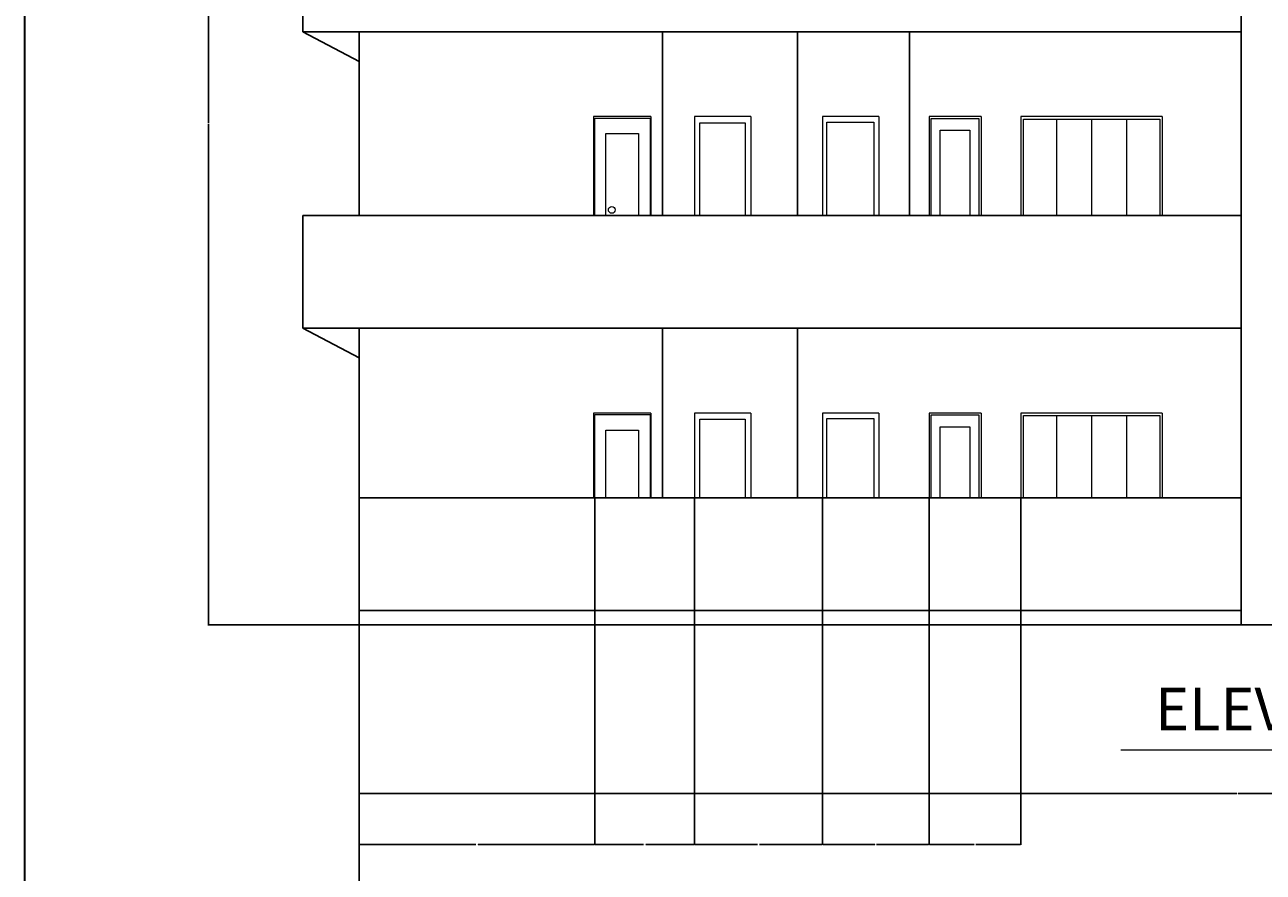
# Model space of a CAD drawing. Units: inches. Extents: x 2120 to 4013, y 1390 to 3019.
# Tile 47 of 59: x 2120 to 2647, y 2364 to 2724. Entities that reach past the tile are written whole.
import ezdxf

# ---------------------------------------------------------------- set-up
doc = ezdxf.new("R2010")
doc.units = ezdxf.units.IN
for name, color, linetype, lineweight in [('A-ANNO-DIMS', 2, 'Continuous', 18), ('A-ANNO-TEXT', 7, 'Continuous', 18), ('A-ANNO-TTLB', 7, 'Continuous', 35), ('A-DOOR', 3, 'Continuous', 18), ('A-ELEV', 7, 'Continuous', 25), ('A-GLAZ', 4, 'Continuous', 18), ('A-WALL-PATT', 252, 'Continuous', 13)]:
    doc.layers.add(name, color=color, linetype=linetype, lineweight=lineweight)
doc.styles.get("Standard").update_dxf_attribs({"font": 'arial.ttf'})
doc.dimstyles.get("Standard").update_dxf_attribs({"dimtxt": 0.18, "dimasz": 0.18, "dimexe": 0.18, "dimexo": 0.0625, "dimgap": 0.09, "dimtad": 0, "dimtih": 1, "dimtoh": 1, "dimdec": 4, "dimzin": 0, "dimdsep": 46, "dimtxsty": 'Standard', "dimcen": 0.09, "dimadec": 0, "dimazin": 0, "dimtfac": 1, "dimtdec": 4, "dimtofl": 0, "dimtmove": 0, "dimatfit": 3, "dimfxl": 1, "dimtolj": 1, "dimtzin": 0, "dimarcsym": 0})

# ---------------------------------------------------------------- blocks, each defined once
blk = doc.blocks.new('*D211')
at = {"layer": 'A-ANNO-DIMS', "color": 0, "lineweight": -2, "transparency": 16777216}
for p, q in [((2262.73, 2352.59), (2262.73, 2397.71)), ((2262.91, 2397.53), (2635.95, 2397.53)), ((3009.55, 2397.53), (2636.52, 2397.53)), ((3009.73, 2352.59), (3009.73, 2397.71))]:
    blk.add_line(p, q, dxfattribs=at)
at = {"layer": 'A-ANNO-DIMS', "color": 0, "transparency": 16777216}
for points in [[(2262.91, 2397.56), (2262.91, 2397.5), (2262.73, 2397.53)], [(3009.55, 2397.56), (3009.55, 2397.5), (3009.73, 2397.53)]]:
    blk.add_solid(points, dxfattribs=at)
at = {"layer": 'Defpoints', "color": 0, "transparency": 16777216}
for p in [(3009.73, 2397.53), (2262.73, 2352.53), (3009.73, 2352.53)]:
    blk.add_point(p, dxfattribs=at)
at = {"layer": 'A-ANNO-DIMS', "color": 0, "transparency": 16777216, "insert": (2636.23, 2397.53), "char_height": 0.18, "attachment_point": 5}
blk.add_mtext('\\A1;747', dxfattribs=at)
blk = doc.blocks.new('*D224')
at = {"layer": 'A-ANNO-DIMS', "color": 0, "lineweight": -2, "transparency": 16777216}
for p, q in [((2238.67, 2895.31), (2198.35, 2895.31)), ((2198.53, 2895.13), (2198.53, 2682.49)), ((2198.53, 2469.49), (2198.53, 2682.13)), ((2262.67, 2469.31), (2198.35, 2469.31))]:
    blk.add_line(p, q, dxfattribs=at)
at = {"layer": 'A-ANNO-DIMS', "color": 0, "transparency": 16777216}
for points in [[(2198.5, 2895.13), (2198.56, 2895.13), (2198.53, 2895.31)], [(2198.5, 2469.49), (2198.56, 2469.49), (2198.53, 2469.31)]]:
    blk.add_solid(points, dxfattribs=at)
at = {"layer": 'Defpoints', "color": 0, "transparency": 16777216}
for p in [(2198.53, 2895.31), (2238.73, 2895.31), (2262.73, 2469.31)]:
    blk.add_point(p, dxfattribs=at)
at = {"layer": 'A-ANNO-DIMS', "color": 0, "transparency": 16777216, "insert": (2198.53, 2682.31), "char_height": 0.18, "attachment_point": 5}
blk.add_mtext('\\A1;426', dxfattribs=at)
blk = doc.blocks.new('*D225')
at = {"layer": 'A-ANNO-DIMS', "color": 0, "lineweight": -2, "transparency": 16777216}
for p, q in [((2262.73, 2523.25), (2262.73, 2375.74)), ((2362.9, 2523.25), (2362.9, 2375.74)), ((2262.91, 2375.92), (2312.36, 2375.92)), ((2362.72, 2375.92), (2313.27, 2375.92))]:
    blk.add_line(p, q, dxfattribs=at)
at = {"layer": 'A-ANNO-DIMS', "color": 0, "transparency": 16777216}
for points in [[(2262.91, 2375.95), (2262.91, 2375.89), (2262.73, 2375.92)], [(2362.72, 2375.95), (2362.72, 2375.89), (2362.9, 2375.92)]]:
    blk.add_solid(points, dxfattribs=at)
at = {"layer": 'Defpoints', "color": 0, "transparency": 16777216}
for p in [(2262.73, 2523.31), (2362.9, 2523.31), (2362.9, 2375.92)]:
    blk.add_point(p, dxfattribs=at)
at = {"layer": 'A-ANNO-DIMS', "color": 0, "transparency": 16777216, "insert": (2312.82, 2375.92), "char_height": 0.18, "attachment_point": 5}
blk.add_mtext('\\A1;100.17', dxfattribs=at)
blk = doc.blocks.new('*D226')
at = {"layer": 'A-ANNO-DIMS', "color": 0, "lineweight": -2, "transparency": 16777216}
for p, q in [((2362.9, 2523.25), (2362.9, 2375.74)), ((2405.3, 2523.25), (2405.3, 2375.74)), ((2363.08, 2375.92), (2383.63, 2375.92)), ((2405.12, 2375.92), (2384.57, 2375.92))]:
    blk.add_line(p, q, dxfattribs=at)
at = {"layer": 'A-ANNO-DIMS', "color": 0, "transparency": 16777216}
for points in [[(2363.08, 2375.95), (2363.08, 2375.89), (2362.9, 2375.92)], [(2405.12, 2375.95), (2405.12, 2375.89), (2405.3, 2375.92)]]:
    blk.add_solid(points, dxfattribs=at)
at = {"layer": 'Defpoints', "color": 0, "transparency": 16777216}
for p in [(2362.9, 2523.31), (2405.3, 2523.31), (2405.3, 2375.92)]:
    blk.add_point(p, dxfattribs=at)
at = {"layer": 'A-ANNO-DIMS', "color": 0, "transparency": 16777216, "insert": (2384.1, 2375.92), "char_height": 0.18, "attachment_point": 5}
blk.add_mtext('\\A1;42.404', dxfattribs=at)
blk = doc.blocks.new('*D227')
at = {"layer": 'A-ANNO-DIMS', "color": 0, "lineweight": -2, "transparency": 16777216}
for p, q in [((2405.3, 2523.25), (2405.3, 2375.74)), ((2459.67, 2523.25), (2459.67, 2375.74)), ((2405.48, 2375.92), (2432.09, 2375.92)), ((2459.49, 2375.92), (2432.88, 2375.92))]:
    blk.add_line(p, q, dxfattribs=at)
at = {"layer": 'A-ANNO-DIMS', "color": 0, "transparency": 16777216}
for points in [[(2405.48, 2375.95), (2405.48, 2375.89), (2405.3, 2375.92)], [(2459.49, 2375.95), (2459.49, 2375.89), (2459.67, 2375.92)]]:
    blk.add_solid(points, dxfattribs=at)
at = {"layer": 'Defpoints', "color": 0, "transparency": 16777216}
for p in [(2405.3, 2523.31), (2459.67, 2523.31), (2459.67, 2375.92)]:
    blk.add_point(p, dxfattribs=at)
at = {"layer": 'A-ANNO-DIMS', "color": 0, "transparency": 16777216, "insert": (2432.49, 2375.92), "char_height": 0.18, "attachment_point": 5}
blk.add_mtext('\\A1;54.37', dxfattribs=at)
blk = doc.blocks.new('*D228')
at = {"layer": 'A-ANNO-DIMS', "color": 0, "lineweight": -2, "transparency": 16777216}
for p, q in [((2459.67, 2523.25), (2459.67, 2375.74)), ((2505.02, 2523.25), (2505.02, 2375.74)), ((2459.85, 2375.92), (2481.95, 2375.92)), ((2504.84, 2375.92), (2482.74, 2375.92))]:
    blk.add_line(p, q, dxfattribs=at)
at = {"layer": 'A-ANNO-DIMS', "color": 0, "transparency": 16777216}
for points in [[(2459.85, 2375.95), (2459.85, 2375.89), (2459.67, 2375.92)], [(2504.84, 2375.95), (2504.84, 2375.89), (2505.02, 2375.92)]]:
    blk.add_solid(points, dxfattribs=at)
at = {"layer": 'Defpoints', "color": 0, "transparency": 16777216}
for p in [(2459.67, 2523.31), (2505.02, 2523.31), (2505.02, 2375.92)]:
    blk.add_point(p, dxfattribs=at)
at = {"layer": 'A-ANNO-DIMS', "color": 0, "transparency": 16777216, "insert": (2482.34, 2375.92), "char_height": 0.18, "attachment_point": 5}
blk.add_mtext('\\A1;45.35', dxfattribs=at)
blk = doc.blocks.new('*D229')
at = {"layer": 'A-ANNO-DIMS', "color": 0, "lineweight": -2, "transparency": 16777216}
for p, q in [((2505.02, 2523.25), (2505.02, 2375.74)), ((2544.14, 2523.25), (2544.14, 2375.74)), ((2505.2, 2375.92), (2524.19, 2375.92)), ((2543.96, 2375.92), (2524.97, 2375.92))]:
    blk.add_line(p, q, dxfattribs=at)
at = {"layer": 'A-ANNO-DIMS', "color": 0, "transparency": 16777216}
for points in [[(2505.2, 2375.95), (2505.2, 2375.89), (2505.02, 2375.92)], [(2543.96, 2375.95), (2543.96, 2375.89), (2544.14, 2375.92)]]:
    blk.add_solid(points, dxfattribs=at)
at = {"layer": 'Defpoints', "color": 0, "transparency": 16777216}
for p in [(2505.02, 2523.31), (2544.14, 2523.31), (2544.14, 2375.92)]:
    blk.add_point(p, dxfattribs=at)
at = {"layer": 'A-ANNO-DIMS', "color": 0, "transparency": 16777216, "insert": (2524.58, 2375.92), "char_height": 0.18, "attachment_point": 5}
blk.add_mtext('\\A1;39.12', dxfattribs=at)

msp = doc.modelspace()

# ---------------------------------------------------------------- hatches: boundary and pattern name
at = {"layer": 'A-WALL-PATT'}
h = msp.add_hatch(dxfattribs=at)
h.set_pattern_fill('ANSI32', color=256)
h.paths.add_polyline_path([(2271.7331, 2343.531), (2283.3788, 2343.531), (2283.3788, 2348.031), (2283.3788, 2352.5306), (2262.7331, 2352.5306), (2262.7331, 2182.638), (2267.2331, 2182.638), (2271.7331, 2182.638), (2271.7331, 2219.031), (2391.7331, 2219.031), (2391.7331, 2214.189), (2393.9831, 2214.189), (2396.2331, 2214.189), (2396.2331, 2219.031), (2420.2331, 2219.031), (2420.2331, 2225.7535), (2417.2197, 2225.7535), (2415.7331, 2225.7535), (2415.7331, 2223.5306), (2271.7331, 2223.5306)])
h.paths.add_polyline_path([(2380.0942, 2352.5306), (2343.3788, 2352.5306), (2343.3788, 2343.531), (2363.2331, 2343.531), (2363.2331, 2288.8489), (2365.4831, 2288.8489), (2367.7331, 2288.8489), (2367.7331, 2343.531), (2380.0942, 2343.531)], flags=17)
h.paths.add_polyline_path([(2432.4339, 2352.5306), (2404.0943, 2352.5306), (2404.0943, 2343.531), (2415.7331, 2343.531), (2415.7331, 2264.0306), (2367.7331, 2264.0306), (2367.7331, 2266.4872), (2363.2331, 2266.4872), (2363.2331, 2259.531), (2367.7331, 2259.531), (2415.7331, 2259.531), (2415.7331, 2255.0658), (2420.2331, 2255.0658), (2420.2331, 2259.531), (2424.5717, 2259.531), (2424.5717, 2261.781), (2424.5717, 2264.0306), (2420.2331, 2264.0306), (2420.2331, 2343.531), (2432.4339, 2343.531)])
h.paths.add_polyline_path([(2508.9115, 2352.5306), (2456.4339, 2352.5306), (2456.4339, 2343.531), (2468.2331, 2343.531), (2468.2331, 2264.0306), (2448.0487, 2264.0306), (2448.0487, 2259.531), (2468.2331, 2259.531), (2468.2331, 2255.5496), (2472.7331, 2255.5496), (2472.7331, 2343.531), (2508.9115, 2343.531)])
h.paths.add_polyline_path([(2637.7331, 2352.5306), (2544.9116, 2352.5306), (2544.9116, 2343.531), (2589.7331, 2343.531), (2633.2331, 2343.531), (2637.7331, 2343.531)])
h.paths.add_polyline_path([(2594.2331, 2343.5306), (2589.7331, 2343.5306), (2589.7331, 2259.5306), (2589.7331, 2252.4915), (2591.9831, 2252.4915), (2594.2331, 2252.4915)])
h.paths.add_polyline_path([(2637.7331, 2223.5306), (2594.2331, 2223.5306), (2594.2331, 2230.1988), (2591.9831, 2230.1988), (2589.7331, 2230.1988), (2589.7331, 2223.5306), (2472.7331, 2223.5306), (2468.2331, 2223.5306), (2468.2331, 2219.031), (2628.7331, 2219.031), (2628.7331, 2138.031), (2637.7331, 2138.031)])
h.paths.add_polyline_path([(3822.6535, 2458.4402), (3874.9468, 2458.4402), (3874.9468, 2476.9866), (3822.6535, 2476.9866)], flags=9)
h.paths.add_polyline_path([(3834.6921, 2781.8174), (3935.9206, 2781.8174), (3935.9206, 2800.3638), (3834.6921, 2800.3638)], flags=9)
h.paths.add_polyline_path([(3832.2843, 2837.9683), (3884.5776, 2837.9683), (3884.5776, 2856.5146), (3832.2843, 2856.5146)], flags=9)
h.paths.add_polyline_path([(3830.9388, 2861.4782), (3956.8958, 2861.4782), (3956.8958, 2880.0245), (3830.9388, 2880.0245)], flags=9)
h.paths.add_polyline_path([(3870.6966, 2352.5752), (3887.9272, 2352.5752), (3887.9272, 2377.3037), (3870.6966, 2377.3037)], flags=9)
h.paths.add_polyline_path([(3289.2701, 2413.161), (3435.2223, 2413.161), (3435.2223, 2450.2538), (3289.2701, 2450.2538)], flags=9)
h.paths.add_polyline_path([(2487.6944, 2414.3601), (2637.8335, 2414.3601), (2637.8335, 2451.4528), (2487.6944, 2451.4528)], flags=9)
h.paths.add_polyline_path([(2567.3724, 1457.9199), (2815.296, 1457.9199), (2815.296, 1495.0127), (2567.3724, 1495.0127)], flags=9)
h.paths.add_polyline_path([(2655.3825, 2093.2363), (2685.9555, 2093.2363), (2685.9555, 2111.8937), (2655.3825, 2111.8937)], flags=9)
h.paths.add_polyline_path([(2543.9218, 1550.6671), (2587.8406, 1550.6671), (2587.8406, 1569.3244), (2543.9218, 1569.3244)], flags=9)
h.paths.add_polyline_path([(2905.1384, 1543.8113), (2949.0572, 1543.8113), (2949.0572, 1562.4686), (2905.1384, 1562.4686)], flags=9)
h.paths.add_polyline_path([(2736.4118, 1702.4736), (2784.2153, 1702.4736), (2784.2153, 1721.1309), (2736.4118, 1721.1309)], flags=9)
h.paths.add_polyline_path([(2912.8666, 1710.4168), (2951.707, 1710.4168), (2951.707, 1729.0741), (2912.8666, 1729.0741)], flags=9)
h.paths.add_polyline_path([(2923.5785, 1763.5038), (2959.7279, 1763.5038), (2959.7279, 1782.1611), (2923.5785, 1782.1611)], flags=9)
h.paths.add_polyline_path([(2925.2114, 1809.6137), (2967.1861, 1809.6137), (2967.1861, 1828.271), (2925.2114, 1828.271)], flags=9)
h.paths.add_polyline_path([(2996.2711, 1878.9003), (2996.2711, 1913.109), (2977.6138, 1913.109), (2977.6138, 1878.9003)], flags=9)
h.paths.add_polyline_path([(2883.0859, 1895.7192), (2927.1855, 1895.7192), (2927.1855, 1914.3766), (2883.0859, 1914.3766)], flags=9)
h.paths.add_polyline_path([(2787.3924, 1810.8013), (2841.0213, 1810.8013), (2841.0213, 1829.4587), (2787.3924, 1829.4587)], flags=9)
h.paths.add_polyline_path([(2775.6399, 2101.7395), (2829.2689, 2101.7395), (2829.2689, 2120.3968), (2775.6399, 2120.3968)], flags=9)
h.paths.add_polyline_path([(2913.0263, 2075.817), (2951.8667, 2075.817), (2951.8667, 2094.4744), (2913.0263, 2094.4744)], flags=9)
h.paths.add_polyline_path([(2929.966, 2133.3669), (2966.1154, 2133.3669), (2966.1154, 2152.0243), (2929.966, 2152.0243)], flags=9)
h.paths.add_polyline_path([(2932.7502, 2182.6088), (2968.8996, 2182.6088), (2968.8996, 2201.2662), (2932.7502, 2201.2662)], flags=9)
h.paths.add_polyline_path([(2996.0681, 2266.3173), (2996.0681, 2300.5261), (2977.4108, 2300.5261), (2977.4108, 2266.3173)], flags=9)
h.paths.add_polyline_path([(2885.1039, 2279.2186), (2929.2035, 2279.2186), (2929.2035, 2297.8759), (2885.1039, 2297.8759)], flags=9)
h.paths.add_polyline_path([(2735.7042, 2218.3197), (2783.5078, 2218.3197), (2783.5078, 2236.9771), (2735.7042, 2236.9771)], flags=9)
h.paths.add_polyline_path([(2635.6049, 2044.0085), (2648.9678, 2044.0085), (2648.9678, 2054.312), (2635.6049, 2054.312)], flags=9)
h.paths.add_polyline_path([(2714.0148, 1923.0473), (2727.3777, 1923.0473), (2727.3777, 1933.3508), (2714.0148, 1933.3508)], flags=9)
h.paths.add_polyline_path([(2709.0345, 1988.1628), (2722.3974, 1988.1628), (2722.3974, 1998.4663), (2709.0345, 1998.4663)], flags=9)
h.paths.add_polyline_path([(2592.8935, 1962.1763), (2606.2564, 1962.1763), (2606.2564, 1972.4799), (2592.8935, 1972.4799)], flags=9)
h.paths.add_polyline_path([(2618.3996, 1985.9724), (2644.1942, 1985.9724), (2644.1942, 1996.2759), (2618.3996, 1996.2759)], flags=9)
h.paths.add_polyline_path([(2601.279, 1920.5869), (2614.6419, 1920.5869), (2614.6419, 1930.8904), (2601.279, 1930.8904)], flags=9)
h.paths.add_polyline_path([(2692.3278, 1932.7645), (2704.5311, 1932.7645), (2704.5311, 1943.0681), (2692.3278, 1943.0681)], flags=9)
h.paths.add_polyline_path([(2311.122, 1672.7318), (2355.0408, 1672.7318), (2355.0408, 1691.3892), (2311.122, 1691.3892)], flags=9)
h.paths.add_polyline_path([(2456.2551, 1632.3198), (2492.4796, 1632.3198), (2492.4796, 1650.9772), (2456.2551, 1650.9772)], flags=9)
h.paths.add_polyline_path([(2401.0766, 1631.4793), (2437.301, 1631.4793), (2437.301, 1650.1367), (2401.0766, 1650.1367)], flags=9)
h.paths.add_polyline_path([(2546.7054, 1700.9235), (2594.509, 1700.9235), (2594.509, 1719.5809), (2546.7054, 1719.5809)], flags=9)
h.paths.add_polyline_path([(2445.4866, 1766.9937), (2497.5261, 1766.9937), (2497.5261, 1785.651), (2445.4866, 1785.651)], flags=9)
h.paths.add_polyline_path([(2287.9992, 1739.7675), (2326.8396, 1739.7675), (2326.8396, 1758.4248), (2287.9992, 1758.4248)], flags=9)
h.paths.add_polyline_path([(2458.5279, 1924.7607), (2510.5675, 1924.7607), (2510.5675, 1943.4181), (2458.5279, 1943.4181)], flags=9)
h.paths.add_polyline_path([(2309.2811, 1902.7642), (2345.4305, 1902.7642), (2345.4305, 1921.4215), (2309.2811, 1921.4215)], flags=9)
h.paths.add_polyline_path([(2490.7554, 2018.9392), (2530.7896, 2018.9392), (2530.7896, 2037.5965), (2490.7554, 2037.5965)], flags=9)
h.paths.add_polyline_path([(2402.143, 2024.7393), (2438.5414, 2024.7393), (2438.5414, 2043.3966), (2402.143, 2043.3966)], flags=9)
h.paths.add_polyline_path([(2287.856, 1931.7926), (2326.6964, 1931.7926), (2326.6964, 1950.4499), (2287.856, 1950.4499)], flags=9)
h.paths.add_polyline_path([(2281.7979, 2193.5771), (2320.6383, 2193.5771), (2320.6383, 2212.2344), (2281.7979, 2212.2344)], flags=25)
h.paths.add_polyline_path([(2484.0754, 2093.892), (2536.115, 2093.892), (2536.115, 2112.5494), (2484.0754, 2112.5494)], flags=9)
h.paths.add_polyline_path([(2624.7948, 2281.8639), (2624.7948, 2311.4137), (2606.1375, 2311.4137), (2606.1375, 2281.8639)], flags=9)
h.paths.add_polyline_path([(2507.5036, 2290.3639), (2541.934, 2290.3639), (2541.934, 2309.0212), (2507.5036, 2309.0212)], flags=9)
h.paths.add_polyline_path([(2423.1076, 2285.2202), (2459.332, 2285.2202), (2459.332, 2303.8776), (2423.1076, 2303.8776)], flags=9)
h.paths.add_polyline_path([(2374.5467, 2289.6272), (2410.7711, 2289.6272), (2410.7711, 2308.2846), (2374.5467, 2308.2846)], flags=25)
h.paths.add_polyline_path([(2277.4907, 2227.5651), (2316.3311, 2227.5651), (2316.3311, 2246.2224), (2277.4907, 2246.2224)], flags=25)
h.paths.add_polyline_path([(2655.3825, 2093.2367), (2685.9555, 2093.2367), (2685.9555, 2111.894), (2655.3825, 2111.894)], flags=9)
h.paths.add_polyline_path([(2543.9217, 1550.6674), (2587.8406, 1550.6674), (2587.8406, 1569.3247), (2543.9217, 1569.3247)], flags=9)
h.paths.add_polyline_path([(2905.1384, 1543.8116), (2949.0572, 1543.8116), (2949.0572, 1562.4689), (2905.1384, 1562.4689)], flags=9)
h.paths.add_polyline_path([(2736.4118, 1702.4739), (2784.2153, 1702.4739), (2784.2153, 1721.1312), (2736.4118, 1721.1312)], flags=9)
h.paths.add_polyline_path([(2912.8666, 1710.4171), (2951.707, 1710.4171), (2951.707, 1729.0744), (2912.8666, 1729.0744)], flags=9)
h.paths.add_polyline_path([(2923.5785, 1763.5041), (2959.7279, 1763.5041), (2959.7279, 1782.1614), (2923.5785, 1782.1614)], flags=9)
h.paths.add_polyline_path([(2925.2114, 1809.614), (2967.1861, 1809.614), (2967.1861, 1828.2713), (2925.2114, 1828.2713)], flags=9)
h.paths.add_polyline_path([(2996.2711, 1878.9006), (2996.2711, 1913.1094), (2977.6137, 1913.1094), (2977.6137, 1878.9006)], flags=9)
h.paths.add_polyline_path([(2883.0859, 1895.7195), (2927.1855, 1895.7195), (2927.1855, 1914.3769), (2883.0859, 1914.3769)], flags=9)
h.paths.add_polyline_path([(2787.3924, 1810.8016), (2841.0213, 1810.8016), (2841.0213, 1829.459), (2787.3924, 1829.459)], flags=9)
h.paths.add_polyline_path([(2775.6399, 2101.7398), (2829.2688, 2101.7398), (2829.2688, 2120.3971), (2775.6399, 2120.3971)], flags=9)
h.paths.add_polyline_path([(2913.0263, 2075.8173), (2951.8667, 2075.8173), (2951.8667, 2094.4747), (2913.0263, 2094.4747)], flags=9)
h.paths.add_polyline_path([(2929.966, 2133.3672), (2966.1154, 2133.3672), (2966.1154, 2152.0246), (2929.966, 2152.0246)], flags=9)
h.paths.add_polyline_path([(2932.7502, 2182.6091), (2968.8996, 2182.6091), (2968.8996, 2201.2665), (2932.7502, 2201.2665)], flags=9)
h.paths.add_polyline_path([(2996.0681, 2266.3176), (2996.0681, 2300.5264), (2977.4108, 2300.5264), (2977.4108, 2266.3176)], flags=9)
h.paths.add_polyline_path([(2885.1039, 2279.2189), (2929.2035, 2279.2189), (2929.2035, 2297.8762), (2885.1039, 2297.8762)], flags=9)
h.paths.add_polyline_path([(2735.7042, 2218.32), (2783.5078, 2218.32), (2783.5078, 2236.9774), (2735.7042, 2236.9774)], flags=9)
h.paths.add_polyline_path([(2635.6048, 2044.0088), (2648.9677, 2044.0088), (2648.9677, 2054.3123), (2635.6048, 2054.3123)], flags=9)
h.paths.add_polyline_path([(2714.0148, 1923.0476), (2727.3777, 1923.0476), (2727.3777, 1933.3511), (2714.0148, 1933.3511)], flags=9)
h.paths.add_polyline_path([(2709.0345, 1988.1631), (2722.3974, 1988.1631), (2722.3974, 1998.4666), (2709.0345, 1998.4666)], flags=9)
h.paths.add_polyline_path([(2592.8935, 1962.1766), (2606.2564, 1962.1766), (2606.2564, 1972.4802), (2592.8935, 1972.4802)], flags=9)
h.paths.add_polyline_path([(2618.3995, 1985.9727), (2644.1942, 1985.9727), (2644.1942, 1996.2762), (2618.3995, 1996.2762)], flags=9)
h.paths.add_polyline_path([(2601.279, 1920.5872), (2614.6419, 1920.5872), (2614.6419, 1930.8908), (2601.279, 1930.8908)], flags=9)
h.paths.add_polyline_path([(2692.3278, 1932.7648), (2704.5311, 1932.7648), (2704.5311, 1943.0684), (2692.3278, 1943.0684)], flags=9)
h.paths.add_polyline_path([(2311.122, 1672.7321), (2355.0408, 1672.7321), (2355.0408, 1691.3895), (2311.122, 1691.3895)], flags=9)
h.paths.add_polyline_path([(2456.2551, 1632.3201), (2492.4795, 1632.3201), (2492.4795, 1650.9775), (2456.2551, 1650.9775)], flags=9)
h.paths.add_polyline_path([(2401.0766, 1631.4796), (2437.301, 1631.4796), (2437.301, 1650.137), (2401.0766, 1650.137)], flags=9)
h.paths.add_polyline_path([(2546.7054, 1700.9238), (2594.509, 1700.9238), (2594.509, 1719.5812), (2546.7054, 1719.5812)], flags=9)
h.paths.add_polyline_path([(2445.4866, 1766.994), (2497.5261, 1766.994), (2497.5261, 1785.6513), (2445.4866, 1785.6513)], flags=9)
h.paths.add_polyline_path([(2287.9992, 1739.7678), (2326.8396, 1739.7678), (2326.8396, 1758.4251), (2287.9992, 1758.4251)], flags=9)
h.paths.add_polyline_path([(2458.5279, 1924.7611), (2510.5675, 1924.7611), (2510.5675, 1943.4184), (2458.5279, 1943.4184)], flags=9)
h.paths.add_polyline_path([(2309.2811, 1902.7645), (2345.4305, 1902.7645), (2345.4305, 1921.4218), (2309.2811, 1921.4218)], flags=9)
h.paths.add_polyline_path([(2490.7554, 2018.9395), (2530.7895, 2018.9395), (2530.7895, 2037.5968), (2490.7554, 2037.5968)], flags=9)
h.paths.add_polyline_path([(2402.143, 2024.7396), (2438.5413, 2024.7396), (2438.5413, 2043.3969), (2402.143, 2043.3969)], flags=9)
h.paths.add_polyline_path([(2287.856, 1931.7929), (2326.6964, 1931.7929), (2326.6964, 1950.4502), (2287.856, 1950.4502)], flags=9)
h.paths.add_polyline_path([(2281.7979, 2193.5774), (2320.6383, 2193.5774), (2320.6383, 2212.2347), (2281.7979, 2212.2347)], flags=25)
h.paths.add_polyline_path([(2484.0754, 2093.8924), (2536.115, 2093.8924), (2536.115, 2112.5497), (2484.0754, 2112.5497)], flags=9)
h.paths.add_polyline_path([(2624.7948, 2281.8642), (2624.7948, 2311.414), (2606.1374, 2311.414), (2606.1374, 2281.8642)], flags=9)
h.paths.add_polyline_path([(2507.5035, 2290.3642), (2541.934, 2290.3642), (2541.934, 2309.0215), (2507.5035, 2309.0215)], flags=9)
h.paths.add_polyline_path([(2423.1075, 2285.2205), (2459.332, 2285.2205), (2459.332, 2303.8779), (2423.1075, 2303.8779)], flags=9)
h.paths.add_polyline_path([(2374.5467, 2289.6275), (2410.7711, 2289.6275), (2410.7711, 2308.2849), (2374.5467, 2308.2849)], flags=25)
h.paths.add_polyline_path([(2277.4907, 2227.5654), (2316.3311, 2227.5654), (2316.3311, 2246.2227), (2277.4907, 2246.2227)], flags=25)
h = msp.add_hatch(dxfattribs=at)
h.set_pattern_fill('ANSI32', color=256)
h.paths.add_polyline_path([(2271.7331, 1980.389), (2262.7331, 1980.389), (2262.7331, 1912.8434), (2267.2331, 1912.8434), (2271.7331, 1912.8434), (2271.7331, 1922.531), (2351.2331, 1922.531), (2351.2331, 1901.4728), (2355.7331, 1901.4728), (2355.7331, 1922.531), (2357.9815, 1922.531), (2357.9815, 1926.5306), (2271.7331, 1926.5306)])
h.paths.add_polyline_path([(2589.2331, 1949.1622), (2584.7331, 1949.1622), (2580.2331, 1949.1622), (2580.2331, 1874.5306), (2355.7331, 1874.5306), (2355.7331, 1880.1922), (2351.2331, 1880.1922), (2351.2331, 1874.5306), (2271.7331, 1874.5306), (2271.7331, 1888.8431), (2262.7331, 1888.8431), (2262.7331, 1842.2909), (2267.2331, 1842.2909), (2271.7331, 1842.2909), (2271.7331, 1865.531), (2415.7331, 1865.531), (2415.7331, 1779.7286), (2420.2331, 1779.7286), (2420.2331, 1865.531), (2589.2331, 1865.531)])
h.paths.add_polyline_path([(2271.7331, 1782.2906), (2262.7331, 1782.2906), (2262.7331, 1711.4639), (2267.2331, 1711.4639), (2271.7331, 1711.4639), (2271.7331, 1738.031), (2420.2331, 1738.031), (2420.2331, 1742.531), (2420.2331, 1747.3376), (2417.9831, 1747.3376), (2415.7331, 1747.3376), (2415.7331, 1742.5306), (2271.7331, 1742.5306)])
h.paths.add_polyline_path([(2271.7331, 1627.031), (2362.3957, 1627.031), (2362.3957, 1629.281), (2362.3957, 1631.5306), (2271.7331, 1631.5306), (2271.7331, 1675.4636), (2262.7331, 1675.4636), (2262.7331, 1581.531), (2405.3032, 1581.531), (2405.3032, 1586.031), (2405.3032, 1590.5306), (2396.2331, 1590.5306), (2396.2331, 1691.4513), (2418.7206, 1691.4513), (2418.7206, 1695.951), (2396.2331, 1695.951), (2391.7331, 1695.951), (2391.7331, 1631.5306), (2386.7425, 1631.5306), (2386.7425, 1629.2806), (2386.7425, 1627.031), (2391.7331, 1627.031), (2391.7331, 1586.1709), (2271.7331, 1586.1709)])
h.paths.add_polyline_path([(2459.6703, 1590.5306), (2429.3032, 1590.5306), (2429.3032, 1581.531), (2459.6703, 1581.531), (2459.6703, 1586.031)])
h.paths.add_polyline_path([(2501.2331, 1590.531), (2501.2331, 1665.0195), (2498.9831, 1665.0195), (2496.7331, 1665.0195), (2496.7331, 1590.5306), (2483.8201, 1590.5306), (2483.8201, 1590.1579), (2483.6704, 1590.1579), (2483.6704, 1581.531), (2505.0196, 1581.531), (2505.0196, 1583.781), (2505.0196, 1586.0306), (2501.2331, 1586.0306)])
h.paths.add_polyline_path([(2544.1361, 1583.781), (2544.1361, 1586.0306), (2527.1368, 1586.0306), (2527.1368, 1583.7806), (2527.1368, 1581.531), (2544.1361, 1581.531)])
h.paths.add_polyline_path([(3822.6535, 2458.4402), (3874.9468, 2458.4402), (3874.9468, 2476.9866), (3822.6535, 2476.9866)], flags=9)
h.paths.add_polyline_path([(3834.6921, 2781.8174), (3935.9206, 2781.8174), (3935.9206, 2800.3638), (3834.6921, 2800.3638)], flags=9)
h.paths.add_polyline_path([(3832.2843, 2837.9683), (3884.5776, 2837.9683), (3884.5776, 2856.5146), (3832.2843, 2856.5146)], flags=9)
h.paths.add_polyline_path([(3830.9388, 2861.4782), (3956.8958, 2861.4782), (3956.8958, 2880.0245), (3830.9388, 2880.0245)], flags=9)
h.paths.add_polyline_path([(3870.6966, 2352.5752), (3887.9272, 2352.5752), (3887.9272, 2377.3037), (3870.6966, 2377.3037)], flags=9)
h.paths.add_polyline_path([(3289.2701, 2413.161), (3435.2223, 2413.161), (3435.2223, 2450.2538), (3289.2701, 2450.2538)], flags=9)
h.paths.add_polyline_path([(2487.6944, 2414.3601), (2637.8335, 2414.3601), (2637.8335, 2451.4528), (2487.6944, 2451.4528)], flags=9)
h.paths.add_polyline_path([(2567.3724, 1457.9199), (2815.296, 1457.9199), (2815.296, 1495.0127), (2567.3724, 1495.0127)], flags=9)
h.paths.add_polyline_path([(2655.3825, 2093.2363), (2685.9555, 2093.2363), (2685.9555, 2111.8937), (2655.3825, 2111.8937)], flags=9)
h.paths.add_polyline_path([(2543.9218, 1550.6671), (2587.8406, 1550.6671), (2587.8406, 1569.3244), (2543.9218, 1569.3244)], flags=9)
h.paths.add_polyline_path([(2905.1384, 1543.8113), (2949.0572, 1543.8113), (2949.0572, 1562.4686), (2905.1384, 1562.4686)], flags=9)
h.paths.add_polyline_path([(2736.4118, 1702.4736), (2784.2153, 1702.4736), (2784.2153, 1721.1309), (2736.4118, 1721.1309)], flags=9)
h.paths.add_polyline_path([(2912.8666, 1710.4168), (2951.707, 1710.4168), (2951.707, 1729.0741), (2912.8666, 1729.0741)], flags=9)
h.paths.add_polyline_path([(2923.5785, 1763.5038), (2959.7279, 1763.5038), (2959.7279, 1782.1611), (2923.5785, 1782.1611)], flags=9)
h.paths.add_polyline_path([(2925.2114, 1809.6137), (2967.1861, 1809.6137), (2967.1861, 1828.271), (2925.2114, 1828.271)], flags=9)
h.paths.add_polyline_path([(2996.2711, 1878.9003), (2996.2711, 1913.109), (2977.6138, 1913.109), (2977.6138, 1878.9003)], flags=9)
h.paths.add_polyline_path([(2883.0859, 1895.7192), (2927.1855, 1895.7192), (2927.1855, 1914.3766), (2883.0859, 1914.3766)], flags=9)
h.paths.add_polyline_path([(2787.3924, 1810.8013), (2841.0213, 1810.8013), (2841.0213, 1829.4587), (2787.3924, 1829.4587)], flags=9)
h.paths.add_polyline_path([(2775.6399, 2101.7395), (2829.2689, 2101.7395), (2829.2689, 2120.3968), (2775.6399, 2120.3968)], flags=9)
h.paths.add_polyline_path([(2913.0263, 2075.817), (2951.8667, 2075.817), (2951.8667, 2094.4744), (2913.0263, 2094.4744)], flags=9)
h.paths.add_polyline_path([(2929.966, 2133.3669), (2966.1154, 2133.3669), (2966.1154, 2152.0243), (2929.966, 2152.0243)], flags=9)
h.paths.add_polyline_path([(2932.7502, 2182.6088), (2968.8996, 2182.6088), (2968.8996, 2201.2662), (2932.7502, 2201.2662)], flags=9)
h.paths.add_polyline_path([(2996.0681, 2266.3173), (2996.0681, 2300.5261), (2977.4108, 2300.5261), (2977.4108, 2266.3173)], flags=9)
h.paths.add_polyline_path([(2885.1039, 2279.2186), (2929.2035, 2279.2186), (2929.2035, 2297.8759), (2885.1039, 2297.8759)], flags=9)
h.paths.add_polyline_path([(2735.7042, 2218.3197), (2783.5078, 2218.3197), (2783.5078, 2236.9771), (2735.7042, 2236.9771)], flags=9)
h.paths.add_polyline_path([(2635.6049, 2044.0085), (2648.9678, 2044.0085), (2648.9678, 2054.312), (2635.6049, 2054.312)], flags=9)
h.paths.add_polyline_path([(2714.0148, 1923.0473), (2727.3777, 1923.0473), (2727.3777, 1933.3508), (2714.0148, 1933.3508)], flags=9)
h.paths.add_polyline_path([(2709.0345, 1988.1628), (2722.3974, 1988.1628), (2722.3974, 1998.4663), (2709.0345, 1998.4663)], flags=9)
h.paths.add_polyline_path([(2592.8935, 1962.1763), (2606.2564, 1962.1763), (2606.2564, 1972.4799), (2592.8935, 1972.4799)], flags=9)
h.paths.add_polyline_path([(2618.3996, 1985.9724), (2644.1942, 1985.9724), (2644.1942, 1996.2759), (2618.3996, 1996.2759)], flags=9)
h.paths.add_polyline_path([(2601.279, 1920.5869), (2614.6419, 1920.5869), (2614.6419, 1930.8904), (2601.279, 1930.8904)], flags=9)
h.paths.add_polyline_path([(2692.3278, 1932.7645), (2704.5311, 1932.7645), (2704.5311, 1943.0681), (2692.3278, 1943.0681)], flags=9)
h.paths.add_polyline_path([(2311.122, 1672.7318), (2355.0408, 1672.7318), (2355.0408, 1691.3892), (2311.122, 1691.3892)], flags=25)
h.paths.add_polyline_path([(2456.2551, 1632.3198), (2492.4796, 1632.3198), (2492.4796, 1650.9772), (2456.2551, 1650.9772)], flags=9)
h.paths.add_polyline_path([(2401.0766, 1631.4793), (2437.301, 1631.4793), (2437.301, 1650.1367), (2401.0766, 1650.1367)], flags=9)
h.paths.add_polyline_path([(2546.7054, 1700.9235), (2594.509, 1700.9235), (2594.509, 1719.5809), (2546.7054, 1719.5809)], flags=9)
h.paths.add_polyline_path([(2445.4866, 1766.9937), (2497.5261, 1766.9937), (2497.5261, 1785.651), (2445.4866, 1785.651)], flags=9)
h.paths.add_polyline_path([(2287.9992, 1739.7675), (2326.8396, 1739.7675), (2326.8396, 1758.4248), (2287.9992, 1758.4248)], flags=24)
h.paths.add_polyline_path([(2458.5279, 1924.7607), (2510.5675, 1924.7607), (2510.5675, 1943.4181), (2458.5279, 1943.4181)], flags=25)
h.paths.add_polyline_path([(2309.2811, 1902.7642), (2345.4305, 1902.7642), (2345.4305, 1921.4215), (2309.2811, 1921.4215)], flags=25)
h.paths.add_polyline_path([(2490.7554, 2018.9392), (2530.7896, 2018.9392), (2530.7896, 2037.5965), (2490.7554, 2037.5965)], flags=9)
h.paths.add_polyline_path([(2402.143, 2024.7393), (2438.5414, 2024.7393), (2438.5414, 2043.3966), (2402.143, 2043.3966)], flags=9)
h.paths.add_polyline_path([(2287.856, 1931.7926), (2326.6964, 1931.7926), (2326.6964, 1950.4499), (2287.856, 1950.4499)], flags=25)
h.paths.add_polyline_path([(2281.7979, 2193.5771), (2320.6383, 2193.5771), (2320.6383, 2212.2344), (2281.7979, 2212.2344)], flags=9)
h.paths.add_polyline_path([(2484.0754, 2093.892), (2536.115, 2093.892), (2536.115, 2112.5494), (2484.0754, 2112.5494)], flags=9)
h.paths.add_polyline_path([(2624.7948, 2281.8639), (2624.7948, 2311.4137), (2606.1375, 2311.4137), (2606.1375, 2281.8639)], flags=9)
h.paths.add_polyline_path([(2507.5036, 2290.3639), (2541.934, 2290.3639), (2541.934, 2309.0212), (2507.5036, 2309.0212)], flags=9)
h.paths.add_polyline_path([(2423.1076, 2285.2202), (2459.332, 2285.2202), (2459.332, 2303.8776), (2423.1076, 2303.8776)], flags=9)
h.paths.add_polyline_path([(2374.5467, 2289.6272), (2410.7711, 2289.6272), (2410.7711, 2308.2846), (2374.5467, 2308.2846)], flags=9)
h.paths.add_polyline_path([(2277.4907, 2227.5651), (2316.3311, 2227.5651), (2316.3311, 2246.2224), (2277.4907, 2246.2224)], flags=9)
h.paths.add_polyline_path([(2655.3825, 2093.2367), (2685.9555, 2093.2367), (2685.9555, 2111.894), (2655.3825, 2111.894)], flags=9)
h.paths.add_polyline_path([(2543.9217, 1550.6674), (2587.8406, 1550.6674), (2587.8406, 1569.3247), (2543.9217, 1569.3247)], flags=9)
h.paths.add_polyline_path([(2905.1384, 1543.8116), (2949.0572, 1543.8116), (2949.0572, 1562.4689), (2905.1384, 1562.4689)], flags=9)
h.paths.add_polyline_path([(2736.4118, 1702.4739), (2784.2153, 1702.4739), (2784.2153, 1721.1312), (2736.4118, 1721.1312)], flags=9)
h.paths.add_polyline_path([(2912.8666, 1710.4171), (2951.707, 1710.4171), (2951.707, 1729.0744), (2912.8666, 1729.0744)], flags=9)
h.paths.add_polyline_path([(2923.5785, 1763.5041), (2959.7279, 1763.5041), (2959.7279, 1782.1614), (2923.5785, 1782.1614)], flags=9)
h.paths.add_polyline_path([(2925.2114, 1809.614), (2967.1861, 1809.614), (2967.1861, 1828.2713), (2925.2114, 1828.2713)], flags=9)
h.paths.add_polyline_path([(2996.2711, 1878.9006), (2996.2711, 1913.1094), (2977.6137, 1913.1094), (2977.6137, 1878.9006)], flags=9)
h.paths.add_polyline_path([(2883.0859, 1895.7195), (2927.1855, 1895.7195), (2927.1855, 1914.3769), (2883.0859, 1914.3769)], flags=9)
h.paths.add_polyline_path([(2787.3924, 1810.8016), (2841.0213, 1810.8016), (2841.0213, 1829.459), (2787.3924, 1829.459)], flags=9)
h.paths.add_polyline_path([(2775.6399, 2101.7398), (2829.2688, 2101.7398), (2829.2688, 2120.3971), (2775.6399, 2120.3971)], flags=9)
h.paths.add_polyline_path([(2913.0263, 2075.8173), (2951.8667, 2075.8173), (2951.8667, 2094.4747), (2913.0263, 2094.4747)], flags=9)
h.paths.add_polyline_path([(2929.966, 2133.3672), (2966.1154, 2133.3672), (2966.1154, 2152.0246), (2929.966, 2152.0246)], flags=9)
h.paths.add_polyline_path([(2932.7502, 2182.6091), (2968.8996, 2182.6091), (2968.8996, 2201.2665), (2932.7502, 2201.2665)], flags=9)
h.paths.add_polyline_path([(2996.0681, 2266.3176), (2996.0681, 2300.5264), (2977.4108, 2300.5264), (2977.4108, 2266.3176)], flags=9)
h.paths.add_polyline_path([(2885.1039, 2279.2189), (2929.2035, 2279.2189), (2929.2035, 2297.8762), (2885.1039, 2297.8762)], flags=9)
h.paths.add_polyline_path([(2735.7042, 2218.32), (2783.5078, 2218.32), (2783.5078, 2236.9774), (2735.7042, 2236.9774)], flags=9)
h.paths.add_polyline_path([(2635.6048, 2044.0088), (2648.9677, 2044.0088), (2648.9677, 2054.3123), (2635.6048, 2054.3123)], flags=9)
h.paths.add_polyline_path([(2714.0148, 1923.0476), (2727.3777, 1923.0476), (2727.3777, 1933.3511), (2714.0148, 1933.3511)], flags=9)
h.paths.add_polyline_path([(2709.0345, 1988.1631), (2722.3974, 1988.1631), (2722.3974, 1998.4666), (2709.0345, 1998.4666)], flags=9)
h.paths.add_polyline_path([(2592.8935, 1962.1766), (2606.2564, 1962.1766), (2606.2564, 1972.4802), (2592.8935, 1972.4802)], flags=9)
h.paths.add_polyline_path([(2618.3995, 1985.9727), (2644.1942, 1985.9727), (2644.1942, 1996.2762), (2618.3995, 1996.2762)], flags=9)
h.paths.add_polyline_path([(2601.279, 1920.5872), (2614.6419, 1920.5872), (2614.6419, 1930.8908), (2601.279, 1930.8908)], flags=9)
h.paths.add_polyline_path([(2692.3278, 1932.7648), (2704.5311, 1932.7648), (2704.5311, 1943.0684), (2692.3278, 1943.0684)], flags=9)
h.paths.add_polyline_path([(2311.122, 1672.7321), (2355.0408, 1672.7321), (2355.0408, 1691.3895), (2311.122, 1691.3895)], flags=25)
h.paths.add_polyline_path([(2456.2551, 1632.3201), (2492.4795, 1632.3201), (2492.4795, 1650.9775), (2456.2551, 1650.9775)], flags=9)
h.paths.add_polyline_path([(2401.0766, 1631.4796), (2437.301, 1631.4796), (2437.301, 1650.137), (2401.0766, 1650.137)], flags=9)
h.paths.add_polyline_path([(2546.7054, 1700.9238), (2594.509, 1700.9238), (2594.509, 1719.5812), (2546.7054, 1719.5812)], flags=9)
h.paths.add_polyline_path([(2445.4866, 1766.994), (2497.5261, 1766.994), (2497.5261, 1785.6513), (2445.4866, 1785.6513)], flags=9)
h.paths.add_polyline_path([(2287.9992, 1739.7678), (2326.8396, 1739.7678), (2326.8396, 1758.4251), (2287.9992, 1758.4251)], flags=24)
h.paths.add_polyline_path([(2458.5279, 1924.7611), (2510.5675, 1924.7611), (2510.5675, 1943.4184), (2458.5279, 1943.4184)], flags=25)
h.paths.add_polyline_path([(2309.2811, 1902.7645), (2345.4305, 1902.7645), (2345.4305, 1921.4218), (2309.2811, 1921.4218)], flags=25)
h.paths.add_polyline_path([(2490.7554, 2018.9395), (2530.7895, 2018.9395), (2530.7895, 2037.5968), (2490.7554, 2037.5968)], flags=9)
h.paths.add_polyline_path([(2402.143, 2024.7396), (2438.5413, 2024.7396), (2438.5413, 2043.3969), (2402.143, 2043.3969)], flags=9)
h.paths.add_polyline_path([(2287.856, 1931.7929), (2326.6964, 1931.7929), (2326.6964, 1950.4502), (2287.856, 1950.4502)], flags=25)
h.paths.add_polyline_path([(2281.7979, 2193.5774), (2320.6383, 2193.5774), (2320.6383, 2212.2347), (2281.7979, 2212.2347)], flags=9)
h.paths.add_polyline_path([(2484.0754, 2093.8924), (2536.115, 2093.8924), (2536.115, 2112.5497), (2484.0754, 2112.5497)], flags=9)
h.paths.add_polyline_path([(2624.7948, 2281.8642), (2624.7948, 2311.414), (2606.1374, 2311.414), (2606.1374, 2281.8642)], flags=9)
h.paths.add_polyline_path([(2507.5035, 2290.3642), (2541.934, 2290.3642), (2541.934, 2309.0215), (2507.5035, 2309.0215)], flags=9)
h.paths.add_polyline_path([(2423.1075, 2285.2205), (2459.332, 2285.2205), (2459.332, 2303.8779), (2423.1075, 2303.8779)], flags=9)
h.paths.add_polyline_path([(2374.5467, 2289.6275), (2410.7711, 2289.6275), (2410.7711, 2308.2849), (2374.5467, 2308.2849)], flags=9)
h.paths.add_polyline_path([(2277.4907, 2227.5654), (2316.3311, 2227.5654), (2316.3311, 2246.2227), (2277.4907, 2246.2227)], flags=9)

# ---------------------------------------------------------------- linework, layer by layer
at = {"layer": 'A-ANNO-TEXT'}
msp.add_line((2586.5728, 2416.1241), (2751.3079, 2416.1241), dxfattribs=at)
at = {"layer": 'A-ANNO-TTLB'}
msp.add_lwpolyline([(2120.4581, 3019.1237), (4012.9334, 3019.1237), (4012.9334, 1390.2222), (2120.4581, 1390.2222)], close=True, dxfattribs=at)
at = {"layer": 'A-DOOR'}
for p, q in [((2362.3957, 2685.3118), (2362.3957, 2643.3118)), ((2386.7425, 2685.3118), (2362.3957, 2685.3118)), ((2362.3957, 2685.3118), (2362.3957, 2643.3118)), ((2386.7425, 2685.3118), (2362.3957, 2685.3118)), ((2386.7425, 2685.3118), (2386.7425, 2643.3118)), ((2386.7425, 2685.3118), (2386.7425, 2643.3118)), ((2505.0196, 2685.3118), (2505.0196, 2643.3118)), ((2527.1368, 2685.3118), (2505.0196, 2685.3118)), ((2505.0196, 2685.3118), (2505.0196, 2643.3118)), ((2527.1368, 2685.3118), (2505.0196, 2685.3118)), ((2527.1368, 2685.3118), (2527.1368, 2643.3118)), ((2527.1368, 2685.3118), (2527.1368, 2643.3118)), ((2362.3957, 2679.3118), (2362.3957, 2643.3118)), ((2386.7425, 2679.3118), (2386.7425, 2643.3118)), ((2505.0196, 2679.3118), (2505.0196, 2643.3118)), ((2527.1368, 2679.3118), (2527.1368, 2643.3118)), ((2362.3957, 2559.3118), (2362.3957, 2523.3118)), ((2386.7425, 2559.3118), (2362.3957, 2559.3118)), ((2386.7425, 2559.3118), (2386.7425, 2523.3118)), ((2505.0196, 2559.3118), (2505.0196, 2523.3118)), ((2527.1368, 2559.3118), (2505.0196, 2559.3118)), ((2527.1368, 2559.3118), (2527.1368, 2523.3118))]:
    msp.add_line(p, q, dxfattribs=at)
for points in [[(2362.8987, 2643.3118), (2362.8987, 2684.6544), (2386.362, 2684.6544), (2386.362, 2643.3118)], [(2505.9355, 2643.3118), (2505.9355, 2684.4713), (2526.1603, 2684.4713), (2526.1603, 2643.3118)], [(2367.5645, 2643.3118), (2367.5645, 2678.0397), (2381.4937, 2678.0397), (2381.4937, 2643.3118)], [(2509.792, 2643.3118), (2509.792, 2679.4761), (2522.4068, 2679.4761), (2522.4068, 2643.3118)], [(2362.8987, 2523.3118), (2362.8987, 2558.6544), (2386.362, 2558.6544), (2386.362, 2523.3118)], [(2505.9355, 2523.3118), (2505.9355, 2558.4713), (2526.1603, 2558.4713), (2526.1603, 2523.3118)], [(2367.5645, 2523.3118), (2367.5645, 2552.0397), (2381.4937, 2552.0397), (2381.4937, 2523.3118)], [(2509.792, 2523.3118), (2509.792, 2553.4761), (2522.4068, 2553.4761), (2522.4068, 2523.3118)]]:
    msp.add_lwpolyline(points, dxfattribs=at)
msp.add_circle((2370.0892, 2645.6184), 1.423, dxfattribs=at)
at = {"layer": 'A-ELEV'}
for p, q in [((2238.7331, 2721.3118), (2238.7331, 2763.3118)), ((2238.7331, 2763.3118), (2238.7331, 2721.3118)), ((2637.7331, 2763.3118), (2637.7331, 2601.3118)), ((2637.7331, 2721.3118), (2238.7331, 2721.3118)), ((2238.7331, 2721.3118), (2262.7331, 2708.6916)), ((2262.7331, 2721.3118), (2262.7331, 2643.3118)), ((2262.7331, 2721.3118), (2262.7331, 2709.3118)), ((2262.7331, 2721.3118), (2262.7331, 2643.3118)), ((2391.7331, 2721.3118), (2391.7331, 2643.3118)), ((2449.0524, 2721.3118), (2449.0524, 2643.3118)), ((2496.7331, 2643.3118), (2496.7331, 2721.3118)), ((2637.7331, 2721.3118), (2637.7331, 2595.3118)), ((2391.7331, 2715.3118), (2391.7331, 2643.3118)), ((2449.0524, 2715.3118), (2449.0524, 2643.3118)), ((2238.7331, 2595.3118), (2238.7331, 2643.3118)), ((2637.7331, 2643.3118), (2238.7331, 2643.3118)), ((2637.7331, 2643.3118), (2637.7331, 2469.3118)), ((2637.7331, 2595.3118), (2238.7331, 2595.3118)), ((2238.7331, 2595.3118), (2262.7331, 2582.6916)), ((2262.7331, 2595.3118), (2262.7331, 2469.3118)), ((2262.7331, 2595.3118), (2262.7331, 2583.3118)), ((2262.7331, 2595.3118), (2262.7331, 2577.3118)), ((2391.7331, 2595.3118), (2391.7331, 2523.3118)), ((2449.0524, 2595.3118), (2449.0524, 2523.3118)), ((2262.7331, 2475.3118), (2262.7331, 2523.3118)), ((2262.7331, 2475.3118), (2262.7331, 2523.3118)), ((2262.7331, 2523.3118), (2496.7331, 2523.3118)), ((2391.7331, 2523.3118), (2391.7331, 2523.3118)), ((2496.7331, 2523.3118), (2637.7331, 2523.3118)), ((2262.7331, 2475.3118), (2262.7331, 2469.3118)), ((2637.7331, 2475.3118), (2262.7331, 2475.3118)), ((2262.7331, 2469.3118), (2637.7331, 2469.3118)), ((2637.7331, 2469.3118), (2715.7331, 2469.3118))]:
    msp.add_line(p, q, dxfattribs=at)
at = {"layer": 'A-GLAZ'}
for p, q in [((2405.3032, 2685.3118), (2405.3032, 2643.3118)), ((2429.3032, 2685.3118), (2405.3032, 2685.3118)), ((2405.3032, 2685.3118), (2405.3032, 2643.3118)), ((2429.3032, 2685.3118), (2405.3032, 2685.3118)), ((2429.3032, 2685.3118), (2429.3032, 2643.3118)), ((2429.3032, 2685.3118), (2429.3032, 2643.3118)), ((2459.6703, 2685.3118), (2459.6703, 2643.3118)), ((2483.6703, 2685.3118), (2459.6703, 2685.3118)), ((2459.6703, 2685.3118), (2459.6703, 2643.3118)), ((2483.6703, 2685.3118), (2459.6703, 2685.3118)), ((2483.6703, 2685.3118), (2483.6703, 2643.3118)), ((2483.6703, 2685.3118), (2483.6703, 2643.3118)), ((2544.1361, 2685.3118), (2544.1361, 2643.3118)), ((2604.1361, 2685.3118), (2544.1361, 2685.3118)), ((2544.1361, 2685.3118), (2544.1361, 2643.3118)), ((2604.1361, 2685.3118), (2544.1361, 2685.3118)), ((2559.2822, 2684.2237), (2559.2822, 2643.3118)), ((2574.1465, 2684.2237), (2574.1465, 2643.3118)), ((2589.0012, 2684.2237), (2589.0012, 2643.3118)), ((2604.1361, 2685.3118), (2604.1361, 2643.3118)), ((2604.1361, 2685.3118), (2604.1361, 2643.3118)), ((2405.3032, 2679.3118), (2405.3032, 2643.3118)), ((2429.3032, 2679.3118), (2429.3032, 2643.3118)), ((2459.6703, 2679.3118), (2459.6703, 2643.3118)), ((2483.6703, 2679.3118), (2483.6703, 2643.3118)), ((2544.1361, 2679.3118), (2544.1361, 2643.3118)), ((2604.1361, 2679.3118), (2604.1361, 2643.3118)), ((2405.3032, 2559.3118), (2405.3032, 2523.3118)), ((2429.3032, 2559.3118), (2405.3032, 2559.3118)), ((2429.3032, 2559.3118), (2429.3032, 2523.3118)), ((2459.6703, 2559.3118), (2459.6703, 2523.3118)), ((2483.6703, 2559.3118), (2459.6703, 2559.3118)), ((2483.6703, 2559.3118), (2483.6703, 2523.3118)), ((2544.1361, 2559.3118), (2544.1361, 2523.3118)), ((2604.1361, 2559.3118), (2544.1361, 2559.3118)), ((2559.2822, 2558.2237), (2559.2822, 2523.3118)), ((2574.1465, 2558.2237), (2574.1465, 2523.3118)), ((2589.0012, 2558.2237), (2589.0012, 2523.3118)), ((2604.1361, 2559.3118), (2604.1361, 2523.3118))]:
    msp.add_line(p, q, dxfattribs=at)
for points in [[(2407.4945, 2643.3118), (2407.4945, 2682.6586), (2426.8868, 2682.6586), (2426.8868, 2643.3118)], [(2461.5996, 2643.3118), (2461.5996, 2682.9767), (2481.6066, 2682.9767), (2481.6066, 2643.3118)], [(2545.1381, 2643.3118), (2545.1381, 2684.2237), (2603.1548, 2684.2237), (2603.1548, 2643.3118)], [(2407.4945, 2523.3118), (2407.4945, 2556.6586), (2426.8868, 2556.6586), (2426.8868, 2523.3118)], [(2461.5996, 2523.3118), (2461.5996, 2556.9767), (2481.6066, 2556.9767), (2481.6066, 2523.3118)], [(2545.1381, 2523.3118), (2545.1381, 2558.2237), (2603.1548, 2558.2237), (2603.1548, 2523.3118)]]:
    msp.add_lwpolyline(points, dxfattribs=at)

# ---------------------------------------------------------------- texts
at = {"layer": 'A-ANNO-TEXT', "insert": (2601.1859, 2442.5081), "char_height": 18, "attachment_point": 1}
msp.add_mtext_dynamic_manual_height_columns('ELEVATION', width=359.82979, gutter_width=12.5, heights=[0], dxfattribs=at)

# ---------------------------------------------------------------- dimensions: what is measured, and where the dimension line sits
at = {"layer": 'A-ANNO-DIMS'}
dim = msp.add_linear_dim(base=(2198.5331, 2895.3118), p1=(2262.7331, 2469.3118), p2=(2238.7331, 2895.3118), angle=90, dimstyle='Standard', override={"dimdec": 0, "dimlfac": 1, "dimrnd": 0, "dimzin": 0, "dimdsep": 46, "dimlunit": 2}, dxfattribs=at)
dim.commit()
dim.dimension.update_dxf_attribs({"geometry": '*D224', "text_midpoint": (2198.5331, 2682.3118)})
for base, p1, p2, override, picture, middle in [((2362.8987, 2375.9241), (2262.7331, 2523.3118), (2362.8987, 2523.3118), {"dimdec": 2, "dimlfac": 1, "dimrnd": 0, "dimzin": 0, "dimdsep": 46, "dimlunit": 2}, '*D225', (2312.8159, 2375.9241)), ((2405.30318, 2375.92406), (2362.8987, 2523.31178), (2405.30318, 2523.31178), {"dimdec": 3, "dimlfac": 1, "dimrnd": 0, "dimzin": 0, "dimdsep": 46, "dimlunit": 2}, '*D226', (2384.10094, 2375.92406)), ((2459.6703, 2375.9241), (2405.3032, 2523.3118), (2459.6703, 2523.3118), {"dimdec": 2, "dimlfac": 1, "dimrnd": 0, "dimzin": 0, "dimdsep": 46, "dimlunit": 2}, '*D227', (2432.4868, 2375.9241)), ((2505.0196, 2375.9241), (2459.6703, 2523.3118), (2505.0196, 2523.3118), {"dimdec": 2, "dimlfac": 1, "dimrnd": 0, "dimzin": 0, "dimdsep": 46, "dimlunit": 2}, '*D228', (2482.345, 2375.9241)), ((2544.1361, 2375.9241), (2505.0196, 2523.3118), (2544.1361, 2523.3118), {"dimdec": 2, "dimlfac": 1, "dimrnd": 0, "dimzin": 0, "dimdsep": 46, "dimlunit": 2}, '*D229', (2524.5778, 2375.9241)), ((3009.7331, 2397.531), (2262.7331, 2352.531), (3009.7331, 2352.531), {"dimdec": 0, "dimlfac": 1, "dimrnd": 0, "dimzin": 0, "dimdsep": 46, "dimlunit": 2}, '*D211', (2636.2331, 2397.531))]:
    dim = msp.add_linear_dim(base=base, p1=p1, p2=p2, dimstyle='Standard', override=override, dxfattribs=at)
    dim.commit()
    dim.dimension.update_dxf_attribs({"geometry": picture, "text_midpoint": middle})

doc.saveas('drawing.dxf')
